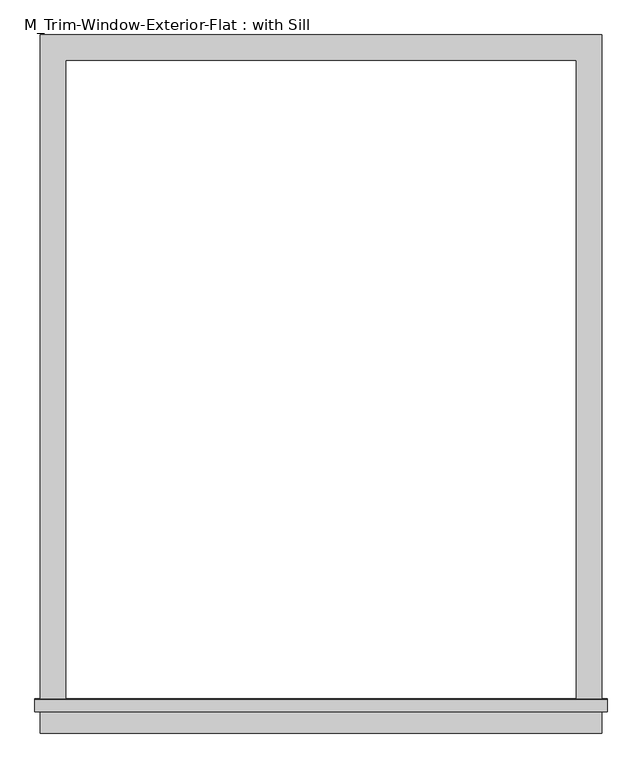
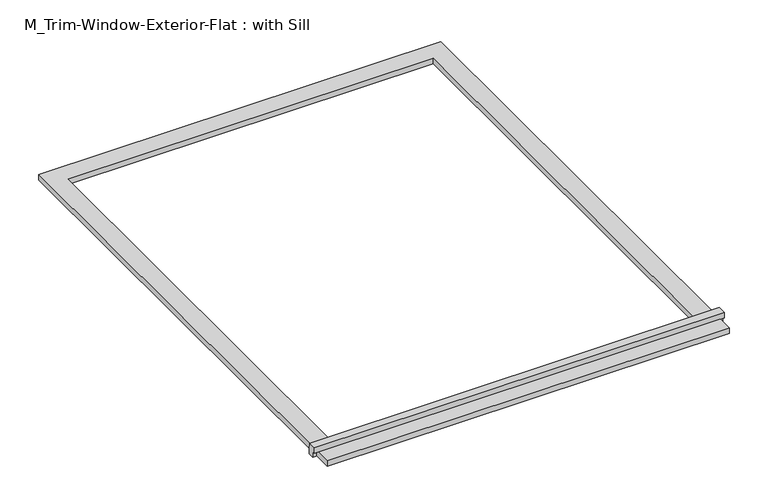
"""IFC4 building model written with IfcOpenShell, lengths in millimetres: proxy geometry, M_Trim-Window-Exterior-Flat : with Sill."""

from ifc_helpers import new_model, si_unit, frame, origin, origin_with_axes, place, context, project, spatial, polyline, outline, extrude, source, transform, mapped, element, save


def m_trim_window_exterior_flat_with_sill_a970d7bf(model_context):
    return source(origin(), model_context, "Body", "SweptSolid", [
        extrude(outline(polyline([(660.0, -1520.4323709), (660.0, -1580.4323709), (-660.0, -1580.4323709), (-660.0, -1520.4323709), (660.0, -1520.4323709)])), origin_with_axes(), (0.0, 0.0, 1.0), 19.05),
        extrude(outline(polyline([(-1530.0, 38.1), (-1502.4580645, 38.1), (-1500.0, 19.05), (-1500.0, 0.0), (-1520.4323709, 0.0), (-1520.4323709, 19.05), (-1530.0, 19.05), (-1530.0, 38.1)])), frame((-672.7, 0.0, 0.0), z_axis=(1.0, 0.0, 0.0), x_axis=(0.0, 1.0, 0.0)), (0.0, 0.0, 1.0), 1345.4),
        extrude(outline(polyline([(-660.0, 60.0), (660.0, 60.0), (660.0, -1500.0), (600.0, -1500.0), (600.0, 0.0), (-600.0, 0.0), (-600.0, -1500.0), (-660.0, -1500.0), (-660.0, 60.0)])), origin_with_axes(), (0.0, 0.0, 1.0), 19.05),
    ])


if __name__ == "__main__":
    model = new_model("IFC4")
    model_context = context("Model", 3, world=origin())
    ifc_project = project(units=[si_unit("LENGTHUNIT", "METRE", prefix="MILLI")], contexts=[model_context])
    site = spatial("IfcSite", under=ifc_project)
    building = spatial("IfcBuilding", under=site)
    placement = place(None, origin())
    m_trim_window_exterior_flat_with_sill_shape = m_trim_window_exterior_flat_with_sill_a970d7bf(model_context)
    element("IfcBuildingElementProxy", 1, Name="M_Trim-Window-Exterior-Flat : with Sill", ObjectType="M_Trim-Window-Exterior-Flat : with Sill", at=placement, inside=building, context=model_context, shape_type="MappedRepresentation", body=[
        mapped(m_trim_window_exterior_flat_with_sill_shape, transform((0.0, 0.0, 0.0), x_axis=(1.0, 0.0, 0.0), y_axis=(0.0, 1.0, 0.0), z_axis=(0.0, 0.0, 1.0))),
    ])
    save(model, "model.ifc")

# Revit data of these elements
# Type "M_Trim-Window-Exterior-Flat : with Sill"
#   Trim Width = 0.19685 ft
#   Trim Thickness_Picture Frame = 0.098425 ft
#   Trim Thickness_with Sill = 0.0625 ft
#   Sill Thickness = 0.098425 ft
#   Opening Width [instance default] = 1.968504 ft
#   Opening Height [instance default] = 2.952756 ft
#   Default Elevation = 3.937008 ft
#   Sill = yes
#   Picture Frame = no
#   Trim Material [instance default] = none
# Element 1 (IfcBuildingElementProxy, "M_Trim-Window-Exterior-Flat : with Sill")
#   Opening Width = 3.937008 ft
#   Opening Height = 4.92126 ft
#   Trim Material = Clad - White
#   Materials on its faces: "Clad - White"
# Materials
#   "Clad - White": class "Wood", colour RGB 242 242 238, transparency 0, Cost = 0
